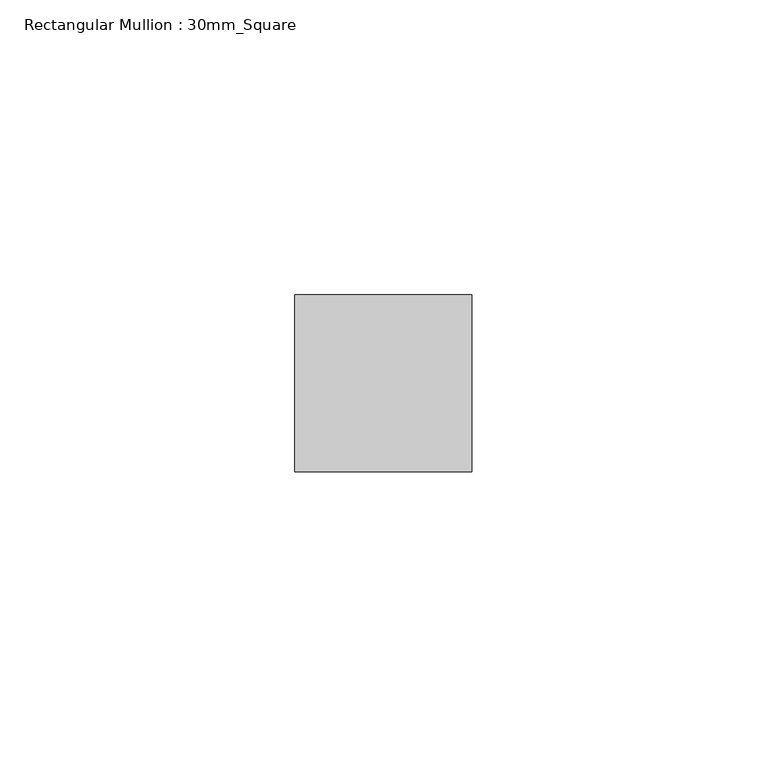
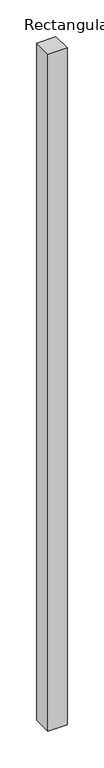
"""IFC4 building model written with IfcOpenShell, lengths in millimetres: member geometry, Rectangular Mullion : 30mm_Square."""

from ifc_helpers import new_model, si_unit, frame, origin, place, context, project, spatial, polyline, outline, extrude, source, transform, mapped, element, save


def rectangular_mullion_30mm_square_82a776c0(model_context):
    return source(origin(), model_context, "Body", "SweptSolid", [
        extrude(outline(polyline([(0.0, 15.0), (0.0, -15.0), (-30.0, -15.0), (-30.0, 15.0), (0.0, 15.0)])), frame((0.0, 0.0, -1121.4666665), z_axis=(0.0, 0.0, 1.0), x_axis=(1.0, 0.0, 0.0)), (0.0, 0.0, 1.0), 1121.4666665),
    ])


if __name__ == "__main__":
    model = new_model("IFC4")
    model_context = context("Model", 3, world=origin())
    ifc_project = project(units=[si_unit("LENGTHUNIT", "METRE", prefix="MILLI")], contexts=[model_context])
    site = spatial("IfcSite", under=ifc_project)
    building = spatial("IfcBuilding", under=site)
    placement = place(None, origin())
    rectangular_mullion_30mm_square_shape = rectangular_mullion_30mm_square_82a776c0(model_context)
    element("IfcMember", 1, ObjectType="Rectangular Mullion : 30mm_Square", at=placement, inside=building, context=model_context, shape_type="MappedRepresentation", body=[
        mapped(rectangular_mullion_30mm_square_shape, transform((0.0, 0.0, 0.0), x_axis=(1.0, 0.0, 0.0), y_axis=(0.0, 1.0, 0.0), z_axis=(0.0, 0.0, 1.0))),
    ])
    save(model, "model.ifc")

# Revit data of these elements
# Type "Rectangular Mullion : 30mm_Square"
#   Keynote = "H11"
#   built-in parameter 1007304 = 0.0984252 (stored number, unit not read)
#   built-in parameter 1007301 = 0.0492126 (stored number, unit not read)
#   built-in parameter 1007300 = 0.0492126 (stored number, unit not read)
# Element 1 (IfcMember, "Rectangular Mullion : 30mm_Square")
#   Materials on its faces: "Aluminium"
# Materials
#   "Aluminium": class "Metal", colour RGB 247 247 247, transparency 0, Description = "Aluminium 6061", Cost = 0
